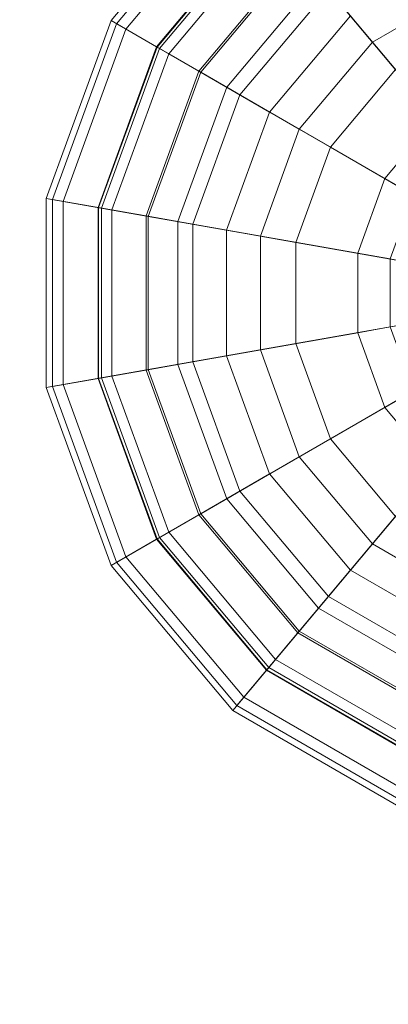
# Model space of a CAD drawing. Units: inches. Extents: x 375 to 1122, y 27 to 1069.
# Tile 13 of 155: x 728.282 to 729.198, y 266.682 to 269.129. Entities that reach past the tile are written whole.
import ezdxf

# ---------------------------------------------------------------- set-up
doc = ezdxf.new("R2010")
doc.units = ezdxf.units.IN
doc.layers.add('Furniture', color=30, linetype='Continuous', lineweight=18)

# ---------------------------------------------------------------- blocks, each defined once
blk = doc.blocks.new('A$C403C54AD')
for points in [[(1.914522, 1.106811, -0.060915), (1.946342, 1.118392, -0.057836), (1.946342, 1.118392, -0.057836), (1.920403, 1.096626, -0.060915)], [(1.920403, 1.096626, -0.060915), (1.946342, 1.118392, -0.057836), (1.946342, 1.118392, -0.057836), (1.929411, 1.089067, -0.060915)], [(1.929411, 1.089067, -0.060915), (1.946342, 1.118392, -0.057836), (1.946342, 1.118392, -0.057836), (1.940462, 1.085044, -0.060915)], [(1.940462, 1.085044, -0.060915), (1.946342, 1.118392, -0.057836), (1.946342, 1.118392, -0.057836), (1.952223, 1.085044, -0.060915)], [(1.972282, 1.096626, -0.060915), (1.946342, 1.118392, -0.057836), (1.946342, 1.118392, -0.057836), (1.978163, 1.106811, -0.060915)], [(1.963274, 1.089067, -0.060915), (1.946342, 1.118392, -0.057836), (1.946342, 1.118392, -0.057836), (1.972282, 1.096626, -0.060915)], [(1.952223, 1.085044, -0.060915), (1.946342, 1.118392, -0.057836), (1.946342, 1.118392, -0.057836), (1.963274, 1.089067, -0.060915)], [(1.927213, 1.111429, 0.032362), (1.936834, 1.114931, 0.024995), (1.938591, 1.111888, 0.024995), (1.930748, 1.105307, 0.032362)], [(1.961937, 1.105307, 0.032362), (1.954094, 1.111888, 0.024995), (1.955851, 1.114931, 0.024995), (1.965472, 1.111429, 0.032362)], [(1.932985, 1.113531, -0.054409), (1.917591, 1.107928, -0.057684), (1.922904, 1.098725, -0.057684), (1.935454, 1.109255, -0.054409)], [(1.957231, 1.109255, -0.054409), (1.969781, 1.098725, -0.057684), (1.975094, 1.107928, -0.057684), (1.9597, 1.113531, -0.054409)], [(1.939522, 1.112669, 0.027913), (1.932456, 1.10674, 0.03455), (1.937279, 1.102693, 0.03455), (1.94189, 1.110681, 0.027913)], [(1.950795, 1.110681, 0.027913), (1.955406, 1.102693, 0.03455), (1.960229, 1.10674, 0.03455), (1.953163, 1.112669, 0.027913)], [(1.929308, 1.112192, 0.03455), (1.923214, 1.109974, 0.043942), (1.927488, 1.102571, 0.043942), (1.932456, 1.10674, 0.03455)], [(1.930748, 1.105307, 0.032362), (1.938591, 1.111888, 0.024995), (1.941283, 1.109629, 0.024995), (1.936164, 1.100762, 0.032362)], [(1.956521, 1.100762, 0.032362), (1.951402, 1.109629, 0.024995), (1.954094, 1.111888, 0.024995), (1.961937, 1.105307, 0.032362)], [(1.960229, 1.10674, 0.03455), (1.965197, 1.102571, 0.043942), (1.969471, 1.109974, 0.043942), (1.963376, 1.112192, 0.03455)], [(1.920572, 1.109013, 0.042594), (1.927213, 1.111429, 0.032362), (1.930748, 1.105307, 0.032362), (1.925335, 1.100764, 0.042594)], [(1.96735, 1.100764, 0.042594), (1.961937, 1.105307, 0.032362), (1.965472, 1.111429, 0.032362), (1.972112, 1.109013, 0.042594)], [(1.937022, 1.110572, -0.051544), (1.935454, 1.109255, -0.054409), (1.939235, 1.106082, -0.054409), (1.940259, 1.107856, -0.051544)], [(1.94189, 1.110681, 0.027913), (1.937279, 1.102693, 0.03455), (1.943195, 1.10054, 0.03455), (1.944796, 1.109623, 0.027913)], [(1.947889, 1.109623, 0.027913), (1.94949, 1.10054, 0.03455), (1.955406, 1.102693, 0.03455), (1.950795, 1.110681, 0.027913)], [(1.952426, 1.107856, -0.051544), (1.95345, 1.106082, -0.054409), (1.957231, 1.109255, -0.054409), (1.955663, 1.110572, -0.051544)], [(1.963564, 1.103941, 0.111475), (1.965922, 1.101963, 0.111475), (1.970361, 1.10965, 0.111475), (1.967468, 1.110703, 0.111475)], [(1.967462, 1.100671, 0.101264), (1.963564, 1.103941, 0.111475), (1.967468, 1.110703, 0.111475), (1.972249, 1.108963, 0.101264)], [(1.965197, 1.102571, 0.043942), (1.96911, 1.099288, 0.061088), (1.974271, 1.108227, 0.061088), (1.969471, 1.109974, 0.043942)], [(1.935454, 1.109255, -0.054409), (1.922904, 1.098725, -0.057684), (1.931044, 1.091895, -0.057684), (1.939235, 1.106082, -0.054409)], [(1.936164, 1.100762, 0.032362), (1.941283, 1.109629, 0.024995), (1.944585, 1.108427, 0.024995), (1.942807, 1.098344, 0.032362)], [(1.944796, 1.109623, 0.027913), (1.943195, 1.10054, 0.03455), (1.94949, 1.10054, 0.03455), (1.947889, 1.109623, 0.027913)], [(1.949878, 1.098344, 0.032362), (1.9481, 1.108427, 0.024995), (1.951402, 1.109629, 0.024995), (1.956521, 1.100762, 0.032362)], [(1.95345, 1.106082, -0.054409), (1.961641, 1.091895, -0.057684), (1.969781, 1.098725, -0.057684), (1.957231, 1.109255, -0.054409)], [(1.965922, 1.101963, 0.111475), (1.96975, 1.098751, 0.102069), (1.975056, 1.107941, 0.102069), (1.970361, 1.10965, 0.111475)], [(1.97146, 1.097316, 0.060603), (1.96735, 1.100764, 0.042594), (1.972112, 1.109013, 0.042594), (1.977153, 1.107178, 0.060603)], [(1.969614, 1.098865, 0.088628), (1.967462, 1.100671, 0.101264), (1.972249, 1.108963, 0.101264), (1.974889, 1.108002, 0.088628)], [(1.942807, 1.098344, 0.032362), (1.944585, 1.108427, 0.024995), (1.9481, 1.108427, 0.024995), (1.949878, 1.098344, 0.032362)], [(1.96911, 1.099288, 0.061088), (1.969614, 1.098865, 0.088628), (1.974889, 1.108002, 0.088628), (1.974271, 1.108227, 0.061088)], [(1.940259, 1.107856, -0.051544), (1.939235, 1.106082, -0.054409), (1.943874, 1.104394, -0.054409), (1.94423, 1.10641, -0.051544)], [(1.948455, 1.10641, -0.051544), (1.948811, 1.104394, -0.054409), (1.95345, 1.106082, -0.054409), (1.952426, 1.107856, -0.051544)], [(1.96975, 1.098751, 0.102069), (1.971977, 1.096882, 0.088845), (1.977788, 1.106947, 0.088845), (1.975056, 1.107941, 0.102069)], [(1.969781, 1.098725, -0.057684), (1.972282, 1.096626, -0.060915), (1.978163, 1.106811, -0.060915), (1.975094, 1.107928, -0.057684)], [(1.932456, 1.10674, 0.03455), (1.927488, 1.102571, 0.043942), (1.934036, 1.097077, 0.043942), (1.937279, 1.102693, 0.03455)], [(1.955406, 1.102693, 0.03455), (1.958649, 1.097077, 0.043942), (1.965197, 1.102571, 0.043942), (1.960229, 1.10674, 0.03455)], [(1.971977, 1.096882, 0.088845), (1.97146, 1.097316, 0.060603), (1.977153, 1.107178, 0.060603), (1.977788, 1.106947, 0.088845)], [(1.94423, 1.10641, -0.051544), (1.943874, 1.104394, -0.054409), (1.948811, 1.104394, -0.054409), (1.948455, 1.10641, -0.051544)], [(1.939235, 1.106082, -0.054409), (1.931044, 1.091895, -0.057684), (1.941029, 1.088261, -0.057684), (1.943874, 1.104394, -0.054409)], [(1.948811, 1.104394, -0.054409), (1.951655, 1.088261, -0.057684), (1.961641, 1.091895, -0.057684), (1.95345, 1.106082, -0.054409)], [(1.925335, 1.100764, 0.042594), (1.930748, 1.105307, 0.032362), (1.936164, 1.100762, 0.032362), (1.932631, 1.094642, 0.042594)], [(1.960054, 1.094642, 0.042594), (1.956521, 1.100762, 0.032362), (1.961937, 1.105307, 0.032362), (1.96735, 1.100764, 0.042594)], [(1.943874, 1.104394, -0.054409), (1.941029, 1.088261, -0.057684), (1.951655, 1.088261, -0.057684), (1.948811, 1.104394, -0.054409)], [(1.925223, 1.100671, 0.101264), (1.929121, 1.103941, 0.111475), (1.935102, 1.098923, 0.111475), (1.932558, 1.094517, 0.101264)], [(1.929121, 1.103941, 0.111475), (1.926763, 1.101963, 0.111475), (1.933563, 1.096257, 0.111475), (1.935102, 1.098923, 0.111475)], [(1.957583, 1.098923, 0.111475), (1.959122, 1.096257, 0.111475), (1.965922, 1.101963, 0.111475), (1.963564, 1.103941, 0.111475)], [(1.960127, 1.094517, 0.101264), (1.957583, 1.098923, 0.111475), (1.963564, 1.103941, 0.111475), (1.967462, 1.100671, 0.101264)], [(1.927488, 1.102571, 0.043942), (1.923575, 1.099288, 0.061088), (1.931482, 1.092653, 0.061088), (1.934036, 1.097077, 0.043942)], [(1.937279, 1.102693, 0.03455), (1.934036, 1.097077, 0.043942), (1.942068, 1.094153, 0.043942), (1.943195, 1.10054, 0.03455)], [(1.94949, 1.10054, 0.03455), (1.950616, 1.094153, 0.043942), (1.958649, 1.097077, 0.043942), (1.955406, 1.102693, 0.03455)], [(1.958649, 1.097077, 0.043942), (1.961203, 1.092653, 0.061088), (1.96911, 1.099288, 0.061088), (1.965197, 1.102571, 0.043942)], [(1.926763, 1.101963, 0.111475), (1.922935, 1.098751, 0.102069), (1.931064, 1.09193, 0.102069), (1.933563, 1.096257, 0.111475)], [(1.959122, 1.096257, 0.111475), (1.96162, 1.09193, 0.102069), (1.96975, 1.098751, 0.102069), (1.965922, 1.101963, 0.111475)], [(1.921225, 1.097316, 0.060603), (1.925335, 1.100764, 0.042594), (1.932631, 1.094642, 0.042594), (1.929948, 1.089997, 0.060603)], [(1.923071, 1.098865, 0.088628), (1.925223, 1.100671, 0.101264), (1.932558, 1.094517, 0.101264), (1.931153, 1.092083, 0.088628)], [(1.932631, 1.094642, 0.042594), (1.936164, 1.100762, 0.032362), (1.942807, 1.098344, 0.032362), (1.94158, 1.091385, 0.042594)], [(1.951105, 1.091385, 0.042594), (1.949878, 1.098344, 0.032362), (1.956521, 1.100762, 0.032362), (1.960054, 1.094642, 0.042594)], [(1.962737, 1.089997, 0.060603), (1.960054, 1.094642, 0.042594), (1.96735, 1.100764, 0.042594), (1.97146, 1.097316, 0.060603)], [(1.961532, 1.092083, 0.088628), (1.960127, 1.094517, 0.101264), (1.967462, 1.100671, 0.101264), (1.969614, 1.098865, 0.088628)], [(1.943195, 1.10054, 0.03455), (1.942068, 1.094153, 0.043942), (1.950616, 1.094153, 0.043942), (1.94949, 1.10054, 0.03455)], [(1.923575, 1.099288, 0.061088), (1.923071, 1.098865, 0.088628), (1.931153, 1.092083, 0.088628), (1.931482, 1.092653, 0.061088)], [(1.932558, 1.094517, 0.101264), (1.935102, 1.098923, 0.111475), (1.942439, 1.096252, 0.111475), (1.941555, 1.091242, 0.101264)], [(1.935102, 1.098923, 0.111475), (1.933563, 1.096257, 0.111475), (1.941904, 1.093221, 0.111475), (1.942439, 1.096252, 0.111475)], [(1.950246, 1.096252, 0.111475), (1.950781, 1.093221, 0.111475), (1.959122, 1.096257, 0.111475), (1.957583, 1.098923, 0.111475)], [(1.95113, 1.091242, 0.101264), (1.950246, 1.096252, 0.111475), (1.957583, 1.098923, 0.111475), (1.960127, 1.094517, 0.101264)], [(1.961203, 1.092653, 0.061088), (1.961532, 1.092083, 0.088628), (1.969614, 1.098865, 0.088628), (1.96911, 1.099288, 0.061088)], [(1.922904, 1.098725, -0.057684), (1.920403, 1.096626, -0.060915), (1.929411, 1.089067, -0.060915), (1.931044, 1.091895, -0.057684)], [(1.922935, 1.098751, 0.102069), (1.920708, 1.096882, 0.088845), (1.929611, 1.089412, 0.088845), (1.931064, 1.09193, 0.102069)], [(1.94158, 1.091385, 0.042594), (1.942807, 1.098344, 0.032362), (1.949878, 1.098344, 0.032362), (1.951105, 1.091385, 0.042594)], [(1.96162, 1.09193, 0.102069), (1.963074, 1.089412, 0.088845), (1.971977, 1.096882, 0.088845), (1.96975, 1.098751, 0.102069)], [(1.961641, 1.091895, -0.057684), (1.963274, 1.089067, -0.060915), (1.972282, 1.096626, -0.060915), (1.969781, 1.098725, -0.057684)], [(1.920708, 1.096882, 0.088845), (1.921225, 1.097316, 0.060603), (1.929948, 1.089997, 0.060603), (1.929611, 1.089412, 0.088845)], [(1.934036, 1.097077, 0.043942), (1.931482, 1.092653, 0.061088), (1.941182, 1.089123, 0.061088), (1.942068, 1.094153, 0.043942)], [(1.950616, 1.094153, 0.043942), (1.951503, 1.089123, 0.061088), (1.961203, 1.092653, 0.061088), (1.958649, 1.097077, 0.043942)], [(1.963074, 1.089412, 0.088845), (1.962737, 1.089997, 0.060603), (1.97146, 1.097316, 0.060603), (1.971977, 1.096882, 0.088845)], [(1.933563, 1.096257, 0.111475), (1.931064, 1.09193, 0.102069), (1.941036, 1.0883, 0.102069), (1.941904, 1.093221, 0.111475)], [(1.941555, 1.091242, 0.101264), (1.942439, 1.096252, 0.111475), (1.950246, 1.096252, 0.111475), (1.95113, 1.091242, 0.101264)], [(1.942439, 1.096252, 0.111475), (1.941904, 1.093221, 0.111475), (1.950781, 1.093221, 0.111475), (1.950246, 1.096252, 0.111475)], [(1.950781, 1.093221, 0.111475), (1.951648, 1.0883, 0.102069), (1.96162, 1.09193, 0.102069), (1.959122, 1.096257, 0.111475)], [(1.929948, 1.089997, 0.060603), (1.932631, 1.094642, 0.042594), (1.94158, 1.091385, 0.042594), (1.940649, 1.086102, 0.060603)], [(1.931153, 1.092083, 0.088628), (1.932558, 1.094517, 0.101264), (1.941555, 1.091242, 0.101264), (1.941067, 1.088475, 0.088628)], [(1.952036, 1.086102, 0.060603), (1.951105, 1.091385, 0.042594), (1.960054, 1.094642, 0.042594), (1.962737, 1.089997, 0.060603)], [(1.951618, 1.088475, 0.088628), (1.95113, 1.091242, 0.101264), (1.960127, 1.094517, 0.101264), (1.961532, 1.092083, 0.088628)], [(1.942068, 1.094153, 0.043942), (1.941182, 1.089123, 0.061088), (1.951503, 1.089123, 0.061088), (1.950616, 1.094153, 0.043942)], [(1.941904, 1.093221, 0.111475), (1.941036, 1.0883, 0.102069), (1.951648, 1.0883, 0.102069), (1.950781, 1.093221, 0.111475)], [(1.931482, 1.092653, 0.061088), (1.931153, 1.092083, 0.088628), (1.941067, 1.088475, 0.088628), (1.941182, 1.089123, 0.061088)], [(1.951503, 1.089123, 0.061088), (1.951618, 1.088475, 0.088628), (1.961532, 1.092083, 0.088628), (1.961203, 1.092653, 0.061088)], [(1.931044, 1.091895, -0.057684), (1.929411, 1.089067, -0.060915), (1.940462, 1.085044, -0.060915), (1.941029, 1.088261, -0.057684)], [(1.931064, 1.09193, 0.102069), (1.929611, 1.089412, 0.088845), (1.940532, 1.085437, 0.088845), (1.941036, 1.0883, 0.102069)], [(1.951648, 1.0883, 0.102069), (1.952153, 1.085437, 0.088845), (1.963074, 1.089412, 0.088845), (1.96162, 1.09193, 0.102069)], [(1.951655, 1.088261, -0.057684), (1.952223, 1.085044, -0.060915), (1.963274, 1.089067, -0.060915), (1.961641, 1.091895, -0.057684)], [(1.940649, 1.086102, 0.060603), (1.94158, 1.091385, 0.042594), (1.951105, 1.091385, 0.042594), (1.952036, 1.086102, 0.060603)], [(1.941067, 1.088475, 0.088628), (1.941555, 1.091242, 0.101264), (1.95113, 1.091242, 0.101264), (1.951618, 1.088475, 0.088628)], [(1.929611, 1.089412, 0.088845), (1.929948, 1.089997, 0.060603), (1.940649, 1.086102, 0.060603), (1.940532, 1.085437, 0.088845)], [(1.952153, 1.085437, 0.088845), (1.952036, 1.086102, 0.060603), (1.962737, 1.089997, 0.060603), (1.963074, 1.089412, 0.088845)], [(1.941182, 1.089123, 0.061088), (1.941067, 1.088475, 0.088628), (1.951618, 1.088475, 0.088628), (1.951503, 1.089123, 0.061088)], [(1.941029, 1.088261, -0.057684), (1.940462, 1.085044, -0.060915), (1.952223, 1.085044, -0.060915), (1.951655, 1.088261, -0.057684)], [(1.941036, 1.0883, 0.102069), (1.940532, 1.085437, 0.088845), (1.952153, 1.085437, 0.088845), (1.951648, 1.0883, 0.102069)], [(1.940532, 1.085437, 0.088845), (1.940649, 1.086102, 0.060603), (1.952036, 1.086102, 0.060603), (1.952153, 1.085437, 0.088845)]]:
    blk.add_3dface(points)
at = {"linetype": 'ByBlock', "invisible_edges": 5}
for points in [[(1.994146, 1.087608, -0.037827), (2.010142, 1.078373, -0.037827), (1.994057, 1.018345, -0.037827), (1.975587, 1.018345, -0.037827)], [(2.023472, 1.070677, -0.05168), (1.994146, 1.087608, -0.042444), (1.975587, 1.018345, -0.042444), (2.009449, 1.018345, -0.05168)]]:
    blk.add_3dface(points, dxfattribs=at)
at = {"linetype": 'ByBlock'}
blk.add_3dface([(1.994146, 1.087608, -0.042444), (1.994146, 1.087608, -0.037827), (1.975587, 1.018345, -0.037827), (1.975587, 1.018345, -0.042444)], dxfattribs=at)

msp = doc.modelspace()

# ---------------------------------------------------------------- block references
at = {"layer": 'Furniture', "xscale": 39.9918517141215, "yscale": 39.9918517141215, "zscale": 39.9918517141215, "rotation": 270}
msp.add_blockref('A$C403C54AD', (684.9549, 346.2875, 0.024), dxfattribs=at)

doc.saveas('drawing.dxf')
